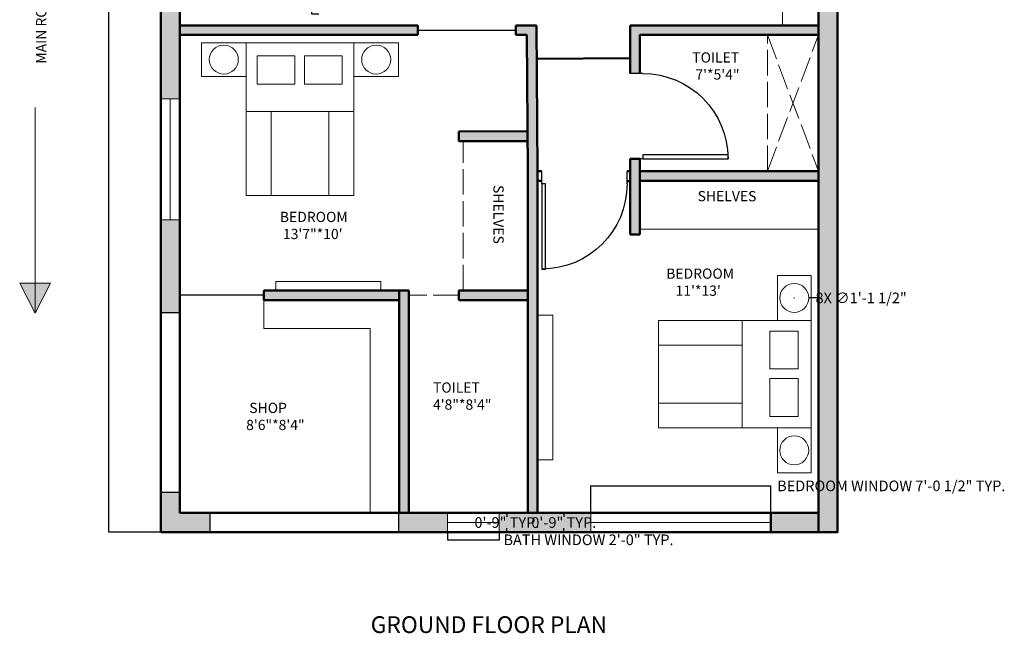
# Model space of a CAD drawing. Units: inches. Extents: x 292 to 1263, y 552 to 1204.
# Tile 1 of 3: x 292 to 754, y 552 to 840. Entities that reach past the tile are written whole.
import ezdxf

# ---------------------------------------------------------------- set-up
doc = ezdxf.new("R2010")
doc.units = ezdxf.units.IN
doc.header["$MEASUREMENT"] = 0
doc.linetypes.add('ACAD_ISO02W100', pattern=[15, 12, -3])
for name, color, linetype, lineweight in [('A-ANNO-DIMS', 2, 'Continuous', 18), ('A-ANNO-SYMB', 7, 'Continuous', 18), ('A-AREA-IDEN', 30, 'Continuous', 18), ('A-DOOR-HIDN', 200, 'ACAD_ISO02W100', 18), ('A-FLOR-CASE', 92, 'Continuous', 18), ('A-FLOR-CASE-HIDN', 92, 'ACAD_ISO02W100', 18), ('A-FLOR-OVHD', 8, 'ACAD_ISO02W100', 18), ('A-WALL-PATT', 22, 'Continuous', 13), ('DOOR', 200, 'Continuous', 25), ('FUR', 92, 'Continuous', 18), ('TEXT', 30, 'Continuous', 18), ('WALL', 22, 'Continuous', 50), ('WIND', 120, 'Continuous', 18)]:
    doc.layers.add(name, color=color, linetype=linetype, lineweight=lineweight)
doc.styles.get("Standard").update_dxf_attribs({"font": 'arial.ttf'})
doc.dimstyles.get("Standard").update_dxf_attribs({"dimtxt": 5, "dimasz": 0.18, "dimexe": 0.18, "dimexo": 0.0625, "dimgap": 0.09, "dimtad": 0, "dimtih": 1, "dimtoh": 1, "dimdec": 0, "dimzin": 0, "dimdsep": 46, "dimlunit": 4, "dimtxsty": 'Standard', "dimcen": 0.09, "dimadec": 0, "dimazin": 0, "dimtfac": 1, "dimtdec": 0, "dimtofl": 0, "dimtmove": 0, "dimatfit": 3, "dimfxl": 1, "dimtolj": 1, "dimtzin": 0, "dimarcsym": 0})

# ---------------------------------------------------------------- blocks, each defined once
blk = doc.blocks.new('*U2')
for p, q in [((0, 0), (0, -6)), ((40, 0), (40, -6))]:
    blk.add_line(p, q)
blk.add_lwpolyline([(0, 0), (0, 40), (1.75, 40), (1.75, 0)], close=True)
blk.add_arc((0, 0), 40, 0, 90)
blk = doc.blocks.new('*D7')
at = {"layer": 'A-ANNO-DIMS', "color": 0, "lineweight": -2, "transparency": 16777216}
for p, q in [((357.91, 1163.64), (333.48, 1163.64)), ((333.66, 1163.46), (333.66, 884.23)), ((333.66, 599.82), (333.66, 879.05)), ((357.91, 599.64), (333.48, 599.64))]:
    blk.add_line(p, q, dxfattribs=at)
at = {"layer": 'A-ANNO-DIMS', "color": 0, "lineweight": 100, "transparency": 16777216}
for points in [[(333.63, 1163.46), (333.69, 1163.46), (333.66, 1163.64)], [(333.63, 599.82), (333.69, 599.82), (333.66, 599.64)]]:
    blk.add_solid(points, dxfattribs=at)
at = {"layer": 'Defpoints', "color": 0, "lineweight": 100, "transparency": 16777216}
for p in [(333.66, 1163.64), (357.97, 1163.64), (357.97, 599.64)]:
    blk.add_point(p, dxfattribs=at)
at = {"layer": 'A-ANNO-DIMS', "color": 0, "transparency": 16777216, "insert": (333.66, 881.64), "char_height": 5, "attachment_point": 5}
blk.add_mtext("\\A1;47'", dxfattribs=at)
blk = doc.blocks.new('BED-DOUBLE')
for p, q in [((39.36, 71.59), (39.36, 21.08)), ((39.36, 71.59), (39.36, 59.89)), ((39.36, 59.89), (0, 59.89)), ((39.36, 32.73), (0, 32.73)), ((39.36, 21.08), (39.36, 32.73))]:
    blk.add_line(p, q)
for points in [[(71.7, 71.59), (55.84, 71.59), (55.84, 92.67), (71.7, 92.67)], [(71.7, 71.59), (0, 71.59), (0, 21.08), (71.7, 21.08)], [(65.61, 66.52), (52.22, 66.52), (52.22, 48.76), (65.61, 48.76)], [(65.61, 44.26), (52.22, 44.26), (52.22, 26.51), (65.61, 26.51)], [(71.7, 0), (55.84, 0), (55.84, 21.08), (71.7, 21.08)]]:
    blk.add_lwpolyline(points, close=True)
for centre in [(63.77, 82.13), (63.77, 10.54)]:
    blk.add_circle(centre, 6.81)
blk = doc.blocks.new('ROAD-DIRECTION')
h = blk.add_hatch(color=256)
h.dxf.hatch_style = 1
h.paths.add_polyline_path([(7.26, 265.02), (0, 250.97), (7.26, 250.97)])
h.paths.add_polyline_path([(7.26, 265.02), (7.26, 250.97), (14.53, 250.97)])
h.paths.add_polyline_path([(14.53, 14.04), (7.26, 14.04), (7.26, 0)])
h.paths.add_polyline_path([(7.26, 14.04), (0, 14.04), (7.26, 0)])
for p, q in [((7.26, 265.02), (0, 250.97)), ((7.26, 168.49), (7.26, 265.02)), ((7.26, 265.02), (14.53, 250.97)), ((0, 250.97), (14.53, 250.97)), ((7.26, 96.52), (7.26, 0)), ((7.26, 0), (0, 14.04)), ((0, 14.04), (14.53, 14.04)), ((7.26, 0), (14.53, 14.04))]:
    blk.add_line(p, q)
blk = doc.blocks.new('WIN-SIDE')
blk.add_line((4.5, 0), (4.5, 56.83))
blk.add_lwpolyline([(9, 56.83), (0, 56.83), (0, 0), (9, 0)], close=True)
blk = doc.blocks.new('WIN-BATH-NARROW')
blk.add_line((0, 4.5), (24.24, 4.5))
blk.add_lwpolyline([(0, 9), (24.24, 9), (24.24, 0), (0, 0)], close=True)
blk = doc.blocks.new('WIN-BEDROOM-WIDE')
blk.add_line((0, 4.5), (84.61, 4.5))
blk.add_lwpolyline([(0, 9), (84.61, 9), (84.61, 0), (0, 0)], close=True)
blk = doc.blocks.new('*D37')
at = {"layer": 'A-ANNO-DIMS', "color": 0, "lineweight": -2, "transparency": 16777216}
for p, q in [((432.33, 866.2), (428.73, 866.2)), ((428.91, 866.02), (428.91, 857.25)), ((428.91, 843.12), (428.91, 851.9)), ((432.33, 842.94), (428.73, 842.94))]:
    blk.add_line(p, q, dxfattribs=at)
at = {"layer": 'A-ANNO-DIMS', "color": 0, "lineweight": 100, "transparency": 16777216}
for points in [[(428.88, 866.02), (428.94, 866.02), (428.91, 866.2)], [(428.88, 843.12), (428.94, 843.12), (428.91, 842.94)]]:
    blk.add_solid(points, dxfattribs=at)
at = {"layer": 'Defpoints', "color": 0, "lineweight": 100, "transparency": 16777216}
for p in [(428.91, 866.2), (432.4, 866.2), (432.4, 842.94)]:
    blk.add_point(p, dxfattribs=at)
at = {"layer": 'A-ANNO-DIMS', "color": 0, "transparency": 16777216, "insert": (428.91, 854.57), "char_height": 5, "attachment_point": 5}
blk.add_mtext('\\A1;LOUNGE CHAIR 1\'-11 1/2" TYP.', dxfattribs=at)
blk = doc.blocks.new('*D41')
at = {"layer": 'A-ANNO-DIMS', "color": 0, "lineweight": -2, "transparency": 16777216}
for p, q in [((492.73, 599.58), (492.73, 595.83)), ((516.97, 599.58), (516.97, 595.83)), ((492.91, 596.01), (516.79, 596.01)), ((516.97, 596.01), (517.15, 596.01))]:
    blk.add_line(p, q, dxfattribs=at)
at = {"layer": 'A-ANNO-DIMS', "color": 0, "lineweight": 100, "transparency": 16777216}
for points in [[(492.91, 596.04), (492.91, 595.98), (492.73, 596.01)], [(516.79, 596.04), (516.79, 595.98), (516.97, 596.01)]]:
    blk.add_solid(points, dxfattribs=at)
at = {"layer": 'Defpoints', "color": 0, "lineweight": 100, "transparency": 16777216}
for p in [(492.73, 599.64), (516.97, 599.64), (516.97, 596.01)]:
    blk.add_point(p, dxfattribs=at)
at = {"layer": 'A-ANNO-DIMS', "color": 0, "transparency": 16777216, "insert": (558.94, 596.01), "char_height": 5, "attachment_point": 5}
blk.add_mtext('\\A1;BATH WINDOW 2\'-0" TYP.', dxfattribs=at)
blk = doc.blocks.new('*D42')
at = {"layer": 'A-ANNO-DIMS', "color": 0, "lineweight": -2, "transparency": 16777216}
for p, q in [((517.03, 608.64), (520.78, 608.64)), ((520.6, 608.46), (520.6, 606.79)), ((520.6, 599.82), (520.6, 601.5)), ((517.03, 599.64), (520.78, 599.64))]:
    blk.add_line(p, q, dxfattribs=at)
at = {"layer": 'A-ANNO-DIMS', "color": 0, "lineweight": 100, "transparency": 16777216}
for points in [[(520.57, 608.46), (520.63, 608.46), (520.6, 608.64)], [(520.57, 599.82), (520.63, 599.82), (520.6, 599.64)]]:
    blk.add_solid(points, dxfattribs=at)
at = {"layer": 'Defpoints', "color": 0, "lineweight": 100, "transparency": 16777216}
for p in [(516.97, 608.64), (520.6, 608.64), (516.97, 599.64)]:
    blk.add_point(p, dxfattribs=at)
at = {"layer": 'A-ANNO-DIMS', "color": 0, "transparency": 16777216, "insert": (520.6, 604.14), "char_height": 5, "attachment_point": 5}
blk.add_mtext('\\A1;0\'-9" TYP.', dxfattribs=at)
blk = doc.blocks.new('*D43')
at = {"layer": 'A-ANNO-DIMS', "color": 0, "lineweight": -2, "transparency": 16777216}
for p, q in [((560.01, 608.71), (560.01, 621.52)), ((560.19, 621.34), (644.45, 621.34)), ((644.63, 608.71), (644.63, 621.52)), ((644.63, 621.34), (644.81, 621.34))]:
    blk.add_line(p, q, dxfattribs=at)
at = {"layer": 'A-ANNO-DIMS', "color": 0, "lineweight": 100, "transparency": 16777216}
for points in [[(560.19, 621.37), (560.19, 621.31), (560.01, 621.34)], [(644.45, 621.37), (644.45, 621.31), (644.63, 621.34)]]:
    blk.add_solid(points, dxfattribs=at)
at = {"layer": 'Defpoints', "color": 0, "lineweight": 100, "transparency": 16777216}
for p in [(644.63, 621.34), (560.01, 608.64), (644.63, 608.64)]:
    blk.add_point(p, dxfattribs=at)
at = {"layer": 'A-ANNO-DIMS', "color": 0, "transparency": 16777216, "insert": (701.16, 621.34), "char_height": 5, "attachment_point": 5}
blk.add_mtext('\\A1;BEDROOM WINDOW 7\'-0 1/2" TYP.', dxfattribs=at)
blk = doc.blocks.new('*D44')
at = {"layer": 'A-ANNO-DIMS', "color": 0, "lineweight": -2, "transparency": 16777216}
for p, q in [((559.95, 608.64), (547.14, 608.64)), ((547.32, 608.46), (547.32, 606.79)), ((547.32, 599.82), (547.32, 601.5)), ((559.95, 599.64), (547.14, 599.64))]:
    blk.add_line(p, q, dxfattribs=at)
at = {"layer": 'A-ANNO-DIMS', "color": 0, "lineweight": 100, "transparency": 16777216}
for points in [[(547.29, 608.46), (547.35, 608.46), (547.32, 608.64)], [(547.29, 599.82), (547.35, 599.82), (547.32, 599.64)]]:
    blk.add_solid(points, dxfattribs=at)
at = {"layer": 'Defpoints', "color": 0, "lineweight": 100, "transparency": 16777216}
for p in [(547.32, 608.64), (560.01, 608.64), (560.01, 599.64)]:
    blk.add_point(p, dxfattribs=at)
at = {"layer": 'A-ANNO-DIMS', "color": 0, "transparency": 16777216, "insert": (547.32, 604.14), "char_height": 5, "attachment_point": 5}
blk.add_mtext('\\A1;0\'-9" TYP.', dxfattribs=at)
blk = doc.blocks.new('*D45')
at = {"layer": 'A-ANNO-DIMS', "color": 0, "lineweight": -2, "transparency": 16777216}
for p, q in [((655.51, 709.62), (655.69, 709.62)), ((655.6, 709.53), (655.6, 709.71)), ((666.49, 709.62), (662.58, 709.62))]:
    blk.add_line(p, q, dxfattribs=at)
at = {"layer": 'A-ANNO-DIMS', "color": 0, "lineweight": 100, "transparency": 16777216}
blk.add_solid([(662.58, 709.65), (662.58, 709.59), (662.4, 709.62)], dxfattribs=at)
at = {"layer": 'Defpoints', "color": 0, "lineweight": 100, "transparency": 16777216}
for p in [(648.79, 709.62), (662.4, 709.62)]:
    blk.add_point(p, dxfattribs=at)
at = {"layer": 'A-ANNO-DIMS', "color": 0, "transparency": 16777216, "insert": (687.01, 709.62), "char_height": 5, "attachment_point": 5}
blk.add_mtext('\\A1;8X ∅1\'-1 1/2"', dxfattribs=at)

msp = doc.modelspace()

# ---------------------------------------------------------------- hatches: boundary and pattern name
at = {"layer": 'A-WALL-PATT'}
h = msp.add_hatch(color=256, dxfattribs=at)
h.dxf.hatch_style = 1
h.paths.add_polyline_path([(675.97, 1154.64), (666.97, 1154.64), (666.97, 599.64), (675.97, 599.64)])
h.paths.add_polyline_path([(666.97, 608.64), (644.63, 608.64), (644.63, 599.64), (666.97, 599.64)])
h.paths.add_polyline_path([(469.97, 713.14), (406.46, 713.14), (406.46, 708.64), (469.97, 708.64)])
h = msp.add_hatch(color=256, dxfattribs=at)
h.dxf.hatch_style = 1
h.paths.add_polyline_path([(366.97, 1038.14), (357.97, 1038.14), (357.97, 1018.14), (366.97, 1018.14)])
h.paths.add_polyline_path([(366.97, 1013.64), (366.97, 1018.14), (357.97, 1018.14), (357.97, 948.4), (366.97, 948.4)])
h.paths.add_polyline_path([(366.97, 891.57), (357.97, 891.57), (357.97, 803.1), (366.97, 803.1), (366.97, 833.14)])
h.paths.add_polyline_path([(366.97, 746.27), (357.97, 746.27), (357.97, 702.82), (366.97, 702.82), (366.97, 708.64)])
h.paths.add_polyline_path([(381.13, 608.64), (367.97, 608.64), (366.97, 608.64), (366.97, 618.29), (357.97, 618.29), (357.97, 599.64), (381.13, 599.64)])
h.paths.add_polyline_path([(492.73, 608.64), (474.47, 608.64), (469.6, 608.64), (469.6, 599.64), (492.73, 599.64)])
h.paths.add_polyline_path([(560.01, 608.64), (516.97, 608.64), (516.97, 599.64), (560.01, 599.64)])
h.paths.add_polyline_path([(474.47, 708.64), (474.47, 713.14), (469.97, 713.14), (469.97, 608.64), (474.47, 608.64)])
h.paths.add_polyline_path([(534.97, 764.64), (534.92, 775.88), (534.43, 837.64), (524.76, 837.64), (524.76, 833.14), (529.97, 833.14), (530.47, 769.14), (530.47, 608.64), (534.97, 608.64)])
h.paths.add_polyline_path([(582.97, 769.14), (582.97, 775.01), (578.47, 775.01), (578.47, 769.14), (578.47, 739.47), (582.97, 739.47), (582.97, 764.64)])
h.paths.add_polyline_path([(666.97, 769.14), (642.97, 769.14), (582.97, 769.14), (582.97, 764.64), (666.97, 764.64)])
h.paths.add_polyline_path([(666.97, 837.64), (578.47, 837.64), (578.47, 816.16), (578.47, 815.01), (582.97, 815.01), (582.97, 816.16), (582.97, 833.14), (666.97, 833.14)])
h.paths.add_polyline_path([(564.59, 912.14), (534.47, 912.14), (534.47, 907.64), (564.59, 907.64)])
h = msp.add_hatch(color=256, dxfattribs=at)
h.dxf.hatch_style = 1
h.paths.add_polyline_path([(478.69, 837.64), (366.97, 837.64), (366.97, 833.14), (478.69, 833.14)])
h = msp.add_hatch(color=256, dxfattribs=at)
h.dxf.hatch_style = 1
h.paths.add_polyline_path([(530.32, 788), (498.01, 787.84), (498.01, 783.2), (530.36, 783.2)])
h = msp.add_hatch(color=256, dxfattribs=at)
h.dxf.hatch_style = 1
h.paths.add_polyline_path([(530.47, 713.14), (498.01, 713.14), (498.01, 708.64), (530.47, 708.64)])

# ---------------------------------------------------------------- linework, layer by layer
at = {"layer": 'A-DOOR-HIDN'}
msp.add_line((498.01, 710.89), (474.47, 710.89), dxfattribs=at)
at = {"layer": 'A-FLOR-CASE'}
for p, q in [((650.02, 907.64), (650.02, 837.64)), ((500.1, 781.16), (500.1, 783.2)), ((582.97, 741.93), (666.97, 741.93)), ((406.46, 695.29), (406.46, 708.64)), ((456.3, 695.29), (406.46, 695.29)), ((456.3, 608.64), (456.3, 695.29))]:
    msp.add_line(p, q, dxfattribs=at)
at = {"layer": 'A-FLOR-CASE-HIDN'}
msp.add_line((500.1, 713.14), (500.1, 781.16), dxfattribs=at)
at = {"layer": 'A-FLOR-OVHD'}
for p, q in [((642.97, 769.14), (642.97, 833.14)), ((642.97, 833.14), (666.97, 769.14)), ((642.97, 769.14), (666.97, 833.14)), ((666.97, 769.14), (642.97, 769.14))]:
    msp.add_line(p, q, dxfattribs=at)
at = {"layer": 'DOOR'}
for p, q in [((478.69, 835.39), (524.76, 835.39)), ((406.46, 710.89), (366.97, 710.89))]:
    msp.add_line(p, q, dxfattribs=at)
for points in [[(366.97, 618.29), (357.97, 618.29), (357.97, 702.82), (366.97, 702.82)], [(381.13, 608.64), (469.6, 608.64), (469.6, 599.64), (381.13, 599.64)]]:
    msp.add_lwpolyline(points, close=True, dxfattribs=at)
at = {"layer": 'FUR'}
for points in [[(412.06, 713.14), (461.42, 713.14), (461.42, 717.29), (412.06, 717.29)], [(534.97, 633.65), (542.25, 633.65), (542.25, 701.47), (534.97, 701.47)]]:
    msp.add_lwpolyline(points, close=True, dxfattribs=at)
at = {"layer": 'WALL'}
for p, q in [((675.97, 599.64), (675.97, 1163.64)), ((666.97, 608.64), (666.97, 1154.64)), ((357.97, 1018.14), (357.97, 599.64)), ((366.97, 1018.14), (366.97, 608.64)), ((366.97, 837.64), (366.97, 1013.64)), ((366.97, 837.64), (478.69, 837.64)), ((478.69, 837.64), (478.69, 833.14)), ((524.76, 837.64), (524.76, 833.14)), ((524.76, 837.64), (534.43, 837.64)), ((534.43, 837.64), (534.97, 769.18)), ((578.47, 837.64), (666.97, 837.64)), ((578.47, 816.16), (578.47, 837.64)), ((366.97, 713.14), (366.97, 833.14)), ((366.97, 833.14), (478.69, 833.14)), ((524.76, 833.14), (529.97, 833.14)), ((529.97, 833.14), (530.47, 769.14)), ((582.97, 833.14), (666.97, 833.14)), ((582.97, 816.16), (582.97, 833.14)), ((578.47, 822.3), (534.56, 821.95)), ((578.47, 816.16), (578.47, 815.01)), ((582.97, 816.16), (582.97, 815.01)), ((498.01, 787.84), (530.32, 788)), ((498.01, 783.2), (498.01, 787.84)), ((530.36, 783.2), (498.01, 783.2)), ((534.97, 764.64), (534.92, 775.88)), ((578.47, 769.14), (578.47, 775.01)), ((582.97, 769.14), (582.97, 775.01)), ((530.47, 769.14), (530.47, 608.64)), ((534.97, 769.18), (537.03, 769.18)), ((578.47, 769.14), (577.03, 769.14)), ((578.47, 739.47), (578.47, 772.07)), ((666.97, 769.14), (582.97, 769.14)), ((666.97, 769.14), (582.97, 769.14)), ((582.97, 769.14), (582.97, 764.64)), ((534.97, 764.64), (534.97, 608.64)), ((534.97, 764.64), (537.03, 764.64)), ((578.47, 764.46), (577.03, 764.46)), ((666.97, 764.64), (582.97, 764.64)), ((582.97, 764.64), (582.97, 739.47)), ((666.97, 608.64), (666.97, 764.64)), ((582.97, 739.47), (578.47, 739.47)), ((406.46, 708.64), (406.46, 713.14)), ((469.97, 608.64), (469.97, 713.14)), ((469.97, 713.14), (474.47, 713.14)), ((474.47, 708.64), (474.47, 713.14)), ((498.01, 713.14), (498.01, 708.64)), ((498.01, 713.14), (530.47, 713.14)), ((474.47, 608.64), (474.47, 708.64)), ((498.01, 708.64), (530.47, 708.64)), ((366.97, 608.64), (666.97, 608.64)), ((469.97, 608.64), (367.97, 608.64)), ((530.47, 608.64), (474.47, 608.64)), ((357.97, 599.64), (675.97, 599.64))]:
    msp.add_line(p, q, dxfattribs=at)
for points in [[(666.97, 1154.64), (675.97, 1154.64), (675.97, 599.64), (666.97, 599.64)], [(644.63, 599.64), (666.97, 599.64), (666.97, 608.64), (644.63, 608.64)]]:
    msp.add_lwpolyline(points, close=True, dxfattribs=at)
for points in [[(582.97, 775.01), (578.47, 775.01)], [(406.46, 713.14), (469.97, 713.14)], [(366.97, 608.64), (366.97, 708.64)], [(406.46, 708.64), (469.97, 708.64)]]:
    msp.add_lwpolyline(points, dxfattribs=at)

# ---------------------------------------------------------------- block references
at = {"layer": 'A-ANNO-SYMB'}
msp.add_blockref('ROAD-DIRECTION', (291.73, 702.52), dxfattribs=at)
at = {"layer": 'DOOR', "xscale": -1}
for p, rotation in [((584.47, 775.01), 270), ((537.03, 763.18), 180)]:
    msp.add_blockref('*U2', p, dxfattribs=dict(at, rotation=rotation))
at = {"layer": 'FUR', "rotation": 89.99999999999996}
msp.add_blockref('BED-DOUBLE', (469.74, 757.77), dxfattribs=at)
at = {"layer": 'FUR'}
msp.add_blockref('BED-DOUBLE', (591.83, 627.49), dxfattribs=at)
at = {"layer": 'WIND'}
for name, p in [('WIN-SIDE', (357.97, 746.27)), ('WIN-BATH-NARROW', (492.73, 599.64)), ('WIN-BEDROOM-WIDE', (560.01, 599.64))]:
    msp.add_blockref(name, p, dxfattribs=at)

# ---------------------------------------------------------------- texts
at = {"layer": 'A-AREA-IDEN', "char_height": 4.805, "attachment_point": 1}
for s, insert in [('TOILET\\P 7\'*5\'4"', (607.68, 824.97)), ('BEDROOM\\P 13\'7"*10\'', (413.93, 750.06)), ("BEDROOM\\P   11'*13'", (595.43, 723.43)), ('TOILET\\P4\'8"*8\'4"', (485.87, 669.94)), (' SHOP\\P8\'6"*8\'4"', (398.1, 660.37))]:
    msp.add_mtext_dynamic_manual_height_columns(s, width=2330.1292, gutter_width=24.03, heights=[0], dxfattribs=dict(at, insert=insert))
at = {"layer": 'TEXT', "char_height": 4.805, "attachment_point": 1}
for s, insert, rotation in [('MAIN ROAD', (299.44, 819.63), 90), ('SHELVES', (519.08, 762.65), 270)]:
    msp.add_mtext_dynamic_manual_height_columns(s, width=2330.1292, gutter_width=24.03, heights=[0], dxfattribs=dict(at, insert=insert, rotation=rotation))
at = {"layer": 'TEXT', "attachment_point": 1}
for s, width, gutter_width, insert, char_height in [('SHELVES', 2330.1292, 24.03, (610.18, 759.82), 4.805), ('GROUND FLOOR PLAN', 3807.3933, 39.26, (456.61, 560.1), 7.8521)]:
    msp.add_mtext_dynamic_manual_height_columns(s, width=width, gutter_width=gutter_width, heights=[0], dxfattribs=dict(at, insert=insert, char_height=char_height))

# ---------------------------------------------------------------- dimensions: what is measured, and where the dimension line sits
at = {"layer": 'A-ANNO-DIMS'}
dim = msp.add_linear_dim(base=(333.66, 1163.64), p1=(357.97, 599.64), p2=(357.97, 1163.64), angle=90, dimstyle='Standard', override={"dimclrd": 0, "dimclre": 0, "dimclrt": 0}, dxfattribs=at)
dim.commit()
dim.dimension.update_dxf_attribs({"geometry": '*D7', "text_midpoint": (333.66, 881.64)})
for base, p1, p2, text, picture, middle in [((428.91, 866.2), (432.4, 842.94), (432.4, 866.2), 'LOUNGE CHAIR <> TYP.', '*D37', (428.91, 854.57)), ((520.6, 608.64), (516.97, 599.64), (516.97, 608.64), '<> TYP.', '*D42', (520.6, 604.14)), ((547.32, 608.64), (560.01, 599.64), (560.01, 608.64), '<> TYP.', '*D44', (547.32, 604.14))]:
    dim = msp.add_linear_dim(base=base, p1=p1, p2=p2, angle=90, text=text, dimstyle='Standard', override={"dimdec": 1, "dimlfac": 1, "dimrnd": 0, "dimzin": 1, "dimdsep": 46, "dimlunit": 4, "dimfrac": 2}, dxfattribs=at)
    dim.commit()
    dim.dimension.update_dxf_attribs({"geometry": picture, "text_midpoint": middle})
dim = msp.add_diameter_dim_2p(p1=(648.79, 709.62), p2=(662.4, 709.62), text='8X <>', dimstyle='Standard', override={"dimdec": 1, "dimlfac": 1, "dimrnd": 0, "dimzin": 1, "dimdsep": 46, "dimlunit": 4, "dimfrac": 2}, dxfattribs=at)
dim.commit()
dim.dimension.update_dxf_attribs({"geometry": '*D45', "text_midpoint": (666.49, 709.62), "dimtype": 163})
for base, p1, p2, text, picture, middle in [((644.63, 621.34), (560.01, 608.64), (644.63, 608.64), 'BEDROOM WINDOW <> TYP.', '*D43', (701.16, 621.34)), ((516.97, 596.01), (492.73, 599.64), (516.97, 599.64), 'BATH WINDOW <> TYP.', '*D41', (558.94, 596.01))]:
    dim = msp.add_linear_dim(base=base, p1=p1, p2=p2, text=text, dimstyle='Standard', override={"dimdec": 1, "dimlfac": 1, "dimrnd": 0, "dimzin": 1, "dimdsep": 46, "dimlunit": 4, "dimfrac": 2}, dxfattribs=at)
    dim.commit()
    dim.dimension.update_dxf_attribs({"geometry": picture, "text_midpoint": middle})

doc.saveas('drawing.dxf')
